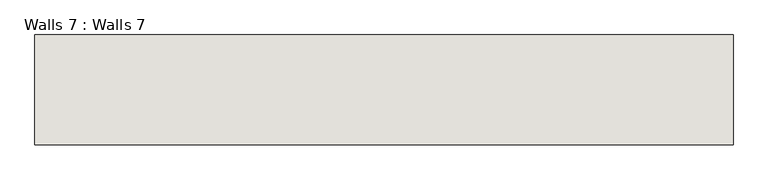
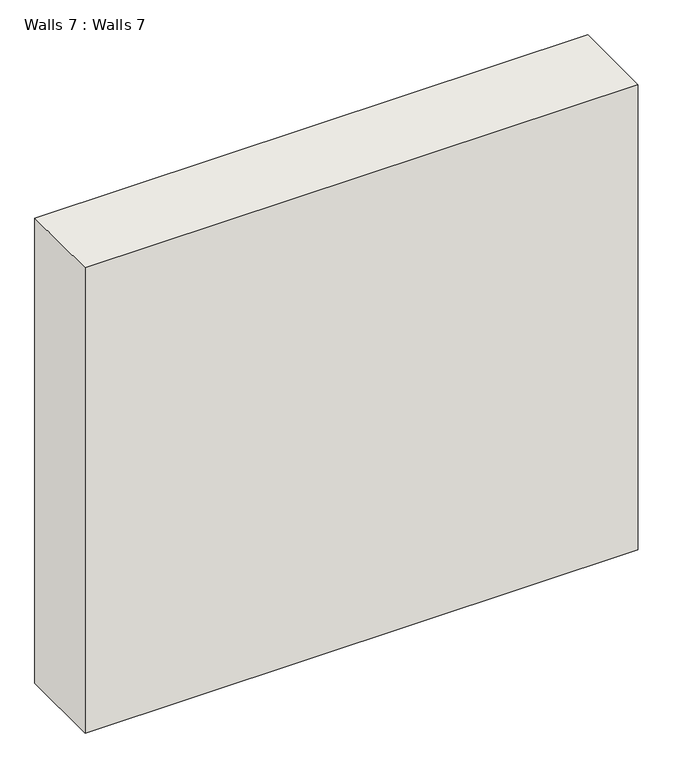
"""IFC4 building model written with IfcOpenShell, lengths in millimetres: wall geometry, Walls 7 : Walls 7."""

from ifc_helpers import new_model, si_unit, frame, origin, place, context, project, spatial, polyline, outline, extrude, source, transform, mapped, element, save


def walls_7_walls_7_d83e4491(model_context):
    return source(origin(), model_context, "Body", "SweptSolid", [
        extrude(outline(polyline([(-10941.4996792, -7792.2759214), (-12313.0996792, -7792.2759214), (-12313.0996792, -7576.9021239), (-10941.4996792, -7576.9021239), (-10941.4996792, -7792.2759214)])), frame((0.0, 0.0, 3756.411322), z_axis=(0.0, 0.0, 1.0), x_axis=(1.0, 0.0, 0.0)), (0.0, 0.0, 1.0), 1219.2),
    ])


if __name__ == "__main__":
    model = new_model("IFC4")
    model_context = context("Model", 3, world=origin())
    ifc_project = project(units=[si_unit("LENGTHUNIT", "METRE", prefix="MILLI")], contexts=[model_context])
    site = spatial("IfcSite", under=ifc_project)
    building = spatial("IfcBuilding", under=site)
    placement = place(None, origin())
    walls_7_walls_7_shape = walls_7_walls_7_d83e4491(model_context)
    element("IfcWall", 1, ObjectType="Walls 7 : Walls 7", at=placement, inside=building, context=model_context, shape_type="MappedRepresentation", body=[
        mapped(walls_7_walls_7_shape, transform((0.0, 0.0, 0.0), x_axis=(1.0, 0.0, 0.0), y_axis=(0.0, 1.0, 0.0), z_axis=(0.0, 0.0, 1.0))),
    ])
    save(model, "model.ifc")

# Revit data of these elements
# Element 1 (IfcWall, "Walls 7 : Walls 7")
#   Materials on its faces: "Default Wall"
# Materials
#   "Default Wall": colour RGB 80 80 80, transparency 0
